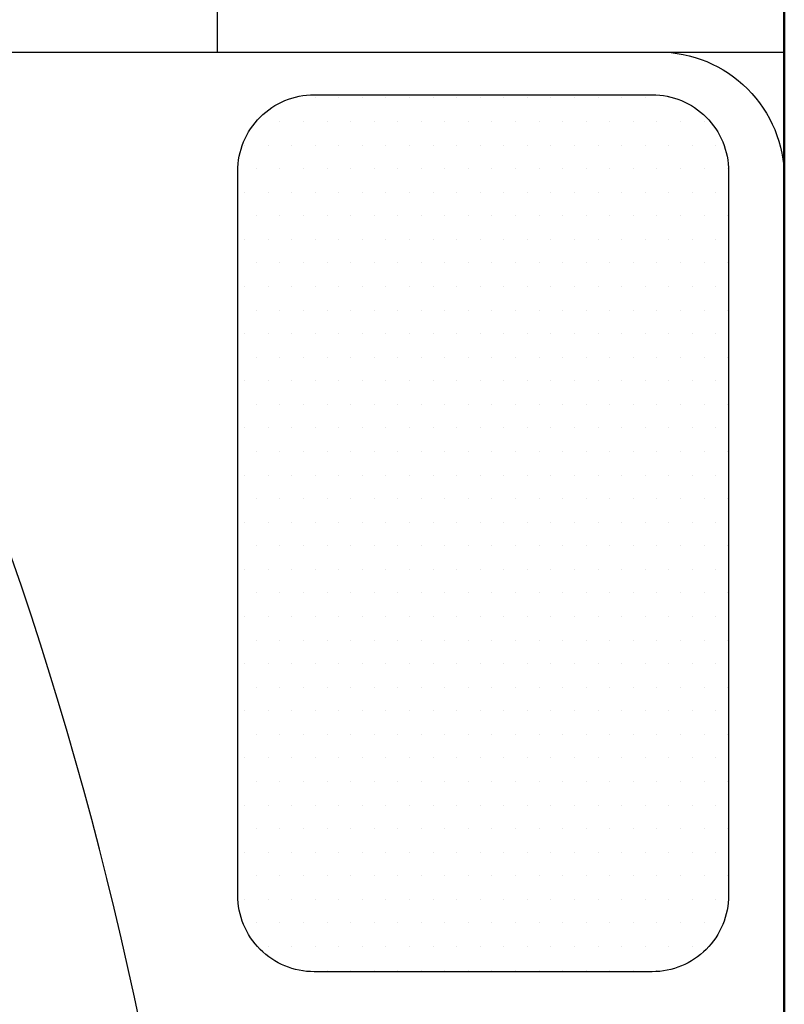
# Model space of a CAD drawing. Units: inches. Extents: x 3064 to 19385, y 846 to 15425.
# Tile 70 of 108: x 6580 to 6604, y 1655 to 1686. Entities that reach past the tile are written whole.
import ezdxf

# ---------------------------------------------------------------- set-up
doc = ezdxf.new("R2010")
doc.units = ezdxf.units.IN
doc.layers.add('A-FLOR-FIXT', color=9, linetype='Continuous', lineweight=18)
doc.layers.add('A-WALL', color=7, linetype='Continuous', lineweight=50)
doc.layers.add('BLOCK', color=6, linetype='Continuous')

# ---------------------------------------------------------------- blocks, each defined once
blk = doc.blocks.new('*X7')
at = {"color": 0}
for p, q in [((266.4375, 457.03125), (266.4375, 457.03125)), ((266.8125, 457.03125), (266.8125, 457.03125)), ((267.1875, 457.03125), (267.1875, 457.03125)), ((267.5625, 457.03125), (267.5625, 457.03125)), ((267.9375, 457.03125), (267.9375, 457.03125)), ((268.3125, 457.03125), (268.3125, 457.03125)), ((268.6875, 457.03125), (268.6875, 457.03125)), ((269.0625, 457.03125), (269.0625, 457.03125)), ((269.4375, 457.03125), (269.4375, 457.03125)), ((269.8125, 457.03125), (269.8125, 457.03125)), ((270.1875, 457.03125), (270.1875, 457.03125)), ((270.5625, 457.03125), (270.5625, 457.03125)), ((270.9375, 457.03125), (270.9375, 457.03125)), ((271.3125, 457.03125), (271.3125, 457.03125)), ((271.6875, 457.03125), (271.6875, 457.03125)), ((272.0625, 457.03125), (272.0625, 457.03125)), ((266.25, 456.9375), (266.25, 456.9375)), ((266.625, 456.9375), (266.625, 456.9375)), ((267, 456.9375), (267, 456.9375)), ((267.375, 456.9375), (267.375, 456.9375)), ((267.75, 456.9375), (267.75, 456.9375)), ((268.125, 456.9375), (268.125, 456.9375)), ((268.5, 456.9375), (268.5, 456.9375)), ((268.875, 456.9375), (268.875, 456.9375)), ((269.25, 456.9375), (269.25, 456.9375)), ((269.625, 456.9375), (269.625, 456.9375)), ((270, 456.9375), (270, 456.9375)), ((270.375, 456.9375), (270.375, 456.9375)), ((270.75, 456.9375), (270.75, 456.9375)), ((271.125, 456.9375), (271.125, 456.9375)), ((271.5, 456.9375), (271.5, 456.9375)), ((271.875, 456.9375), (271.875, 456.9375)), ((272.25, 456.9375), (272.25, 456.9375)), ((266.0625, 456.84375), (266.0625, 456.84375)), ((266.4375, 456.84375), (266.4375, 456.84375)), ((266.8125, 456.84375), (266.8125, 456.84375)), ((267.1875, 456.84375), (267.1875, 456.84375)), ((267.5625, 456.84375), (267.5625, 456.84375)), ((267.9375, 456.84375), (267.9375, 456.84375)), ((268.3125, 456.84375), (268.3125, 456.84375)), ((268.6875, 456.84375), (268.6875, 456.84375)), ((269.0625, 456.84375), (269.0625, 456.84375)), ((269.4375, 456.84375), (269.4375, 456.84375)), ((269.8125, 456.84375), (269.8125, 456.84375)), ((270.1875, 456.84375), (270.1875, 456.84375)), ((270.5625, 456.84375), (270.5625, 456.84375)), ((270.9375, 456.84375), (270.9375, 456.84375)), ((271.3125, 456.84375), (271.3125, 456.84375)), ((271.6875, 456.84375), (271.6875, 456.84375)), ((272.0625, 456.84375), (272.0625, 456.84375)), ((272.4375, 456.84375), (272.4375, 456.84375)), ((266.25, 456.75), (266.25, 456.75)), ((266.625, 456.75), (266.625, 456.75)), ((267, 456.75), (267, 456.75)), ((267.375, 456.75), (267.375, 456.75)), ((267.75, 456.75), (267.75, 456.75)), ((268.125, 456.75), (268.125, 456.75)), ((268.5, 456.75), (268.5, 456.75)), ((268.875, 456.75), (268.875, 456.75)), ((269.25, 456.75), (269.25, 456.75)), ((269.625, 456.75), (269.625, 456.75)), ((270, 456.75), (270, 456.75)), ((270.375, 456.75), (270.375, 456.75)), ((270.75, 456.75), (270.75, 456.75)), ((271.125, 456.75), (271.125, 456.75)), ((271.5, 456.75), (271.5, 456.75)), ((271.875, 456.75), (271.875, 456.75)), ((272.25, 456.75), (272.25, 456.75)), ((272.625, 456.75), (272.625, 456.75)), ((266.0625, 456.65625), (266.0625, 456.65625)), ((266.4375, 456.65625), (266.4375, 456.65625)), ((266.8125, 456.65625), (266.8125, 456.65625)), ((267.1875, 456.65625), (267.1875, 456.65625)), ((267.5625, 456.65625), (267.5625, 456.65625)), ((267.9375, 456.65625), (267.9375, 456.65625)), ((268.3125, 456.65625), (268.3125, 456.65625)), ((268.6875, 456.65625), (268.6875, 456.65625)), ((269.0625, 456.65625), (269.0625, 456.65625)), ((269.4375, 456.65625), (269.4375, 456.65625)), ((269.8125, 456.65625), (269.8125, 456.65625)), ((270.1875, 456.65625), (270.1875, 456.65625)), ((270.5625, 456.65625), (270.5625, 456.65625)), ((270.9375, 456.65625), (270.9375, 456.65625)), ((271.3125, 456.65625), (271.3125, 456.65625)), ((271.6875, 456.65625), (271.6875, 456.65625)), ((272.0625, 456.65625), (272.0625, 456.65625)), ((272.4375, 456.65625), (272.4375, 456.65625)), ((265.875, 456.5625), (265.875, 456.5625)), ((266.25, 456.5625), (266.25, 456.5625)), ((266.625, 456.5625), (266.625, 456.5625)), ((267, 456.5625), (267, 456.5625)), ((267.375, 456.5625), (267.375, 456.5625)), ((267.75, 456.5625), (267.75, 456.5625)), ((268.125, 456.5625), (268.125, 456.5625)), ((268.5, 456.5625), (268.5, 456.5625)), ((268.875, 456.5625), (268.875, 456.5625)), ((269.25, 456.5625), (269.25, 456.5625)), ((269.625, 456.5625), (269.625, 456.5625)), ((270, 456.5625), (270, 456.5625)), ((270.375, 456.5625), (270.375, 456.5625)), ((270.75, 456.5625), (270.75, 456.5625)), ((271.125, 456.5625), (271.125, 456.5625)), ((271.5, 456.5625), (271.5, 456.5625)), ((271.875, 456.5625), (271.875, 456.5625)), ((272.25, 456.5625), (272.25, 456.5625)), ((272.625, 456.5625), (272.625, 456.5625)), ((266.0625, 456.46875), (266.0625, 456.46875)), ((266.4375, 456.46875), (266.4375, 456.46875)), ((266.8125, 456.46875), (266.8125, 456.46875)), ((267.1875, 456.46875), (267.1875, 456.46875)), ((267.5625, 456.46875), (267.5625, 456.46875)), ((267.9375, 456.46875), (267.9375, 456.46875)), ((268.3125, 456.46875), (268.3125, 456.46875)), ((268.6875, 456.46875), (268.6875, 456.46875)), ((269.0625, 456.46875), (269.0625, 456.46875)), ((269.4375, 456.46875), (269.4375, 456.46875)), ((269.8125, 456.46875), (269.8125, 456.46875)), ((270.1875, 456.46875), (270.1875, 456.46875)), ((270.5625, 456.46875), (270.5625, 456.46875)), ((270.9375, 456.46875), (270.9375, 456.46875)), ((271.3125, 456.46875), (271.3125, 456.46875)), ((271.6875, 456.46875), (271.6875, 456.46875)), ((272.0625, 456.46875), (272.0625, 456.46875)), ((272.4375, 456.46875), (272.4375, 456.46875)), ((272.8125, 456.46875), (272.8125, 456.46875)), ((265.875, 456.375), (265.875, 456.375)), ((266.25, 456.375), (266.25, 456.375)), ((266.625, 456.375), (266.625, 456.375)), ((267, 456.375), (267, 456.375)), ((267.375, 456.375), (267.375, 456.375)), ((267.75, 456.375), (267.75, 456.375)), ((268.125, 456.375), (268.125, 456.375)), ((268.5, 456.375), (268.5, 456.375)), ((268.875, 456.375), (268.875, 456.375)), ((269.25, 456.375), (269.25, 456.375)), ((269.625, 456.375), (269.625, 456.375)), ((270, 456.375), (270, 456.375)), ((270.375, 456.375), (270.375, 456.375)), ((270.75, 456.375), (270.75, 456.375)), ((271.125, 456.375), (271.125, 456.375)), ((271.5, 456.375), (271.5, 456.375)), ((271.875, 456.375), (271.875, 456.375)), ((272.25, 456.375), (272.25, 456.375)), ((272.625, 456.375), (272.625, 456.375)), ((266.0625, 456.28125), (266.0625, 456.28125)), ((266.4375, 456.28125), (266.4375, 456.28125)), ((266.8125, 456.28125), (266.8125, 456.28125)), ((267.1875, 456.28125), (267.1875, 456.28125)), ((267.5625, 456.28125), (267.5625, 456.28125)), ((267.9375, 456.28125), (267.9375, 456.28125)), ((268.3125, 456.28125), (268.3125, 456.28125)), ((268.6875, 456.28125), (268.6875, 456.28125)), ((269.0625, 456.28125), (269.0625, 456.28125)), ((269.4375, 456.28125), (269.4375, 456.28125)), ((269.8125, 456.28125), (269.8125, 456.28125)), ((270.1875, 456.28125), (270.1875, 456.28125)), ((270.5625, 456.28125), (270.5625, 456.28125)), ((270.9375, 456.28125), (270.9375, 456.28125)), ((271.3125, 456.28125), (271.3125, 456.28125)), ((271.6875, 456.28125), (271.6875, 456.28125)), ((272.0625, 456.28125), (272.0625, 456.28125)), ((272.4375, 456.28125), (272.4375, 456.28125)), ((272.8125, 456.28125), (272.8125, 456.28125)), ((265.875, 456.1875), (265.875, 456.1875)), ((266.25, 456.1875), (266.25, 456.1875)), ((266.625, 456.1875), (266.625, 456.1875)), ((267, 456.1875), (267, 456.1875)), ((267.375, 456.1875), (267.375, 456.1875)), ((267.75, 456.1875), (267.75, 456.1875)), ((268.125, 456.1875), (268.125, 456.1875)), ((268.5, 456.1875), (268.5, 456.1875)), ((268.875, 456.1875), (268.875, 456.1875)), ((269.25, 456.1875), (269.25, 456.1875)), ((269.625, 456.1875), (269.625, 456.1875)), ((270, 456.1875), (270, 456.1875)), ((270.375, 456.1875), (270.375, 456.1875)), ((270.75, 456.1875), (270.75, 456.1875)), ((271.125, 456.1875), (271.125, 456.1875)), ((271.5, 456.1875), (271.5, 456.1875)), ((271.875, 456.1875), (271.875, 456.1875)), ((272.25, 456.1875), (272.25, 456.1875)), ((272.625, 456.1875), (272.625, 456.1875)), ((266.0625, 456.09375), (266.0625, 456.09375)), ((266.4375, 456.09375), (266.4375, 456.09375)), ((266.8125, 456.09375), (266.8125, 456.09375)), ((267.1875, 456.09375), (267.1875, 456.09375)), ((267.5625, 456.09375), (267.5625, 456.09375)), ((267.9375, 456.09375), (267.9375, 456.09375)), ((268.3125, 456.09375), (268.3125, 456.09375)), ((268.6875, 456.09375), (268.6875, 456.09375)), ((269.0625, 456.09375), (269.0625, 456.09375)), ((269.4375, 456.09375), (269.4375, 456.09375)), ((269.8125, 456.09375), (269.8125, 456.09375)), ((270.1875, 456.09375), (270.1875, 456.09375)), ((270.5625, 456.09375), (270.5625, 456.09375)), ((270.9375, 456.09375), (270.9375, 456.09375)), ((271.3125, 456.09375), (271.3125, 456.09375)), ((271.6875, 456.09375), (271.6875, 456.09375)), ((272.0625, 456.09375), (272.0625, 456.09375)), ((272.4375, 456.09375), (272.4375, 456.09375)), ((272.8125, 456.09375), (272.8125, 456.09375)), ((265.875, 456), (265.875, 456)), ((266.25, 456), (266.25, 456)), ((266.625, 456), (266.625, 456)), ((267, 456), (267, 456)), ((267.375, 456), (267.375, 456)), ((267.75, 456), (267.75, 456)), ((268.125, 456), (268.125, 456)), ((268.5, 456), (268.5, 456)), ((268.875, 456), (268.875, 456)), ((269.25, 456), (269.25, 456)), ((269.625, 456), (269.625, 456)), ((270, 456), (270, 456)), ((270.375, 456), (270.375, 456)), ((270.75, 456), (270.75, 456)), ((271.125, 456), (271.125, 456)), ((271.5, 456), (271.5, 456)), ((271.875, 456), (271.875, 456)), ((272.25, 456), (272.25, 456)), ((272.625, 456), (272.625, 456)), ((266.0625, 455.90625), (266.0625, 455.90625)), ((266.4375, 455.90625), (266.4375, 455.90625)), ((266.8125, 455.90625), (266.8125, 455.90625)), ((267.1875, 455.90625), (267.1875, 455.90625)), ((267.5625, 455.90625), (267.5625, 455.90625)), ((267.9375, 455.90625), (267.9375, 455.90625)), ((268.3125, 455.90625), (268.3125, 455.90625)), ((268.6875, 455.90625), (268.6875, 455.90625)), ((269.0625, 455.90625), (269.0625, 455.90625)), ((269.4375, 455.90625), (269.4375, 455.90625)), ((269.8125, 455.90625), (269.8125, 455.90625)), ((270.1875, 455.90625), (270.1875, 455.90625)), ((270.5625, 455.90625), (270.5625, 455.90625)), ((270.9375, 455.90625), (270.9375, 455.90625)), ((271.3125, 455.90625), (271.3125, 455.90625)), ((271.6875, 455.90625), (271.6875, 455.90625)), ((272.0625, 455.90625), (272.0625, 455.90625)), ((272.4375, 455.90625), (272.4375, 455.90625)), ((272.8125, 455.90625), (272.8125, 455.90625)), ((265.875, 455.8125), (265.875, 455.8125)), ((266.25, 455.8125), (266.25, 455.8125)), ((266.625, 455.8125), (266.625, 455.8125)), ((267, 455.8125), (267, 455.8125)), ((267.375, 455.8125), (267.375, 455.8125)), ((267.75, 455.8125), (267.75, 455.8125)), ((268.125, 455.8125), (268.125, 455.8125)), ((268.5, 455.8125), (268.5, 455.8125)), ((268.875, 455.8125), (268.875, 455.8125)), ((269.25, 455.8125), (269.25, 455.8125)), ((269.625, 455.8125), (269.625, 455.8125)), ((270, 455.8125), (270, 455.8125)), ((270.375, 455.8125), (270.375, 455.8125)), ((270.75, 455.8125), (270.75, 455.8125)), ((271.125, 455.8125), (271.125, 455.8125)), ((271.5, 455.8125), (271.5, 455.8125)), ((271.875, 455.8125), (271.875, 455.8125)), ((272.25, 455.8125), (272.25, 455.8125)), ((272.625, 455.8125), (272.625, 455.8125)), ((266.0625, 455.71875), (266.0625, 455.71875)), ((266.4375, 455.71875), (266.4375, 455.71875)), ((266.8125, 455.71875), (266.8125, 455.71875)), ((267.1875, 455.71875), (267.1875, 455.71875)), ((267.5625, 455.71875), (267.5625, 455.71875)), ((267.9375, 455.71875), (267.9375, 455.71875)), ((268.3125, 455.71875), (268.3125, 455.71875)), ((268.6875, 455.71875), (268.6875, 455.71875)), ((269.0625, 455.71875), (269.0625, 455.71875)), ((269.4375, 455.71875), (269.4375, 455.71875)), ((269.8125, 455.71875), (269.8125, 455.71875)), ((270.1875, 455.71875), (270.1875, 455.71875)), ((270.5625, 455.71875), (270.5625, 455.71875)), ((270.9375, 455.71875), (270.9375, 455.71875)), ((271.3125, 455.71875), (271.3125, 455.71875)), ((271.6875, 455.71875), (271.6875, 455.71875)), ((272.0625, 455.71875), (272.0625, 455.71875)), ((272.4375, 455.71875), (272.4375, 455.71875)), ((272.8125, 455.71875), (272.8125, 455.71875)), ((265.875, 455.625), (265.875, 455.625)), ((266.25, 455.625), (266.25, 455.625)), ((266.625, 455.625), (266.625, 455.625)), ((267, 455.625), (267, 455.625)), ((267.375, 455.625), (267.375, 455.625)), ((267.75, 455.625), (267.75, 455.625)), ((268.125, 455.625), (268.125, 455.625)), ((268.5, 455.625), (268.5, 455.625)), ((268.875, 455.625), (268.875, 455.625)), ((269.25, 455.625), (269.25, 455.625)), ((269.625, 455.625), (269.625, 455.625)), ((270, 455.625), (270, 455.625)), ((270.375, 455.625), (270.375, 455.625)), ((270.75, 455.625), (270.75, 455.625)), ((271.125, 455.625), (271.125, 455.625)), ((271.5, 455.625), (271.5, 455.625)), ((271.875, 455.625), (271.875, 455.625)), ((272.25, 455.625), (272.25, 455.625)), ((272.625, 455.625), (272.625, 455.625)), ((266.0625, 455.53125), (266.0625, 455.53125)), ((266.4375, 455.53125), (266.4375, 455.53125)), ((266.8125, 455.53125), (266.8125, 455.53125)), ((267.1875, 455.53125), (267.1875, 455.53125)), ((267.5625, 455.53125), (267.5625, 455.53125)), ((267.9375, 455.53125), (267.9375, 455.53125)), ((268.3125, 455.53125), (268.3125, 455.53125)), ((268.6875, 455.53125), (268.6875, 455.53125)), ((269.0625, 455.53125), (269.0625, 455.53125)), ((269.4375, 455.53125), (269.4375, 455.53125)), ((269.8125, 455.53125), (269.8125, 455.53125)), ((270.1875, 455.53125), (270.1875, 455.53125)), ((270.5625, 455.53125), (270.5625, 455.53125)), ((270.9375, 455.53125), (270.9375, 455.53125)), ((271.3125, 455.53125), (271.3125, 455.53125)), ((271.6875, 455.53125), (271.6875, 455.53125)), ((272.0625, 455.53125), (272.0625, 455.53125)), ((272.4375, 455.53125), (272.4375, 455.53125)), ((272.8125, 455.53125), (272.8125, 455.53125)), ((265.875, 455.4375), (265.875, 455.4375)), ((266.25, 455.4375), (266.25, 455.4375)), ((266.625, 455.4375), (266.625, 455.4375)), ((267, 455.4375), (267, 455.4375)), ((267.375, 455.4375), (267.375, 455.4375)), ((267.75, 455.4375), (267.75, 455.4375)), ((268.125, 455.4375), (268.125, 455.4375)), ((268.5, 455.4375), (268.5, 455.4375)), ((268.875, 455.4375), (268.875, 455.4375)), ((269.25, 455.4375), (269.25, 455.4375)), ((269.625, 455.4375), (269.625, 455.4375)), ((270, 455.4375), (270, 455.4375)), ((270.375, 455.4375), (270.375, 455.4375)), ((270.75, 455.4375), (270.75, 455.4375)), ((271.125, 455.4375), (271.125, 455.4375)), ((271.5, 455.4375), (271.5, 455.4375)), ((271.875, 455.4375), (271.875, 455.4375)), ((272.25, 455.4375), (272.25, 455.4375)), ((272.625, 455.4375), (272.625, 455.4375)), ((266.0625, 455.34375), (266.0625, 455.34375)), ((266.4375, 455.34375), (266.4375, 455.34375)), ((266.8125, 455.34375), (266.8125, 455.34375)), ((267.1875, 455.34375), (267.1875, 455.34375)), ((267.5625, 455.34375), (267.5625, 455.34375)), ((267.9375, 455.34375), (267.9375, 455.34375)), ((268.3125, 455.34375), (268.3125, 455.34375)), ((268.6875, 455.34375), (268.6875, 455.34375)), ((269.0625, 455.34375), (269.0625, 455.34375)), ((269.4375, 455.34375), (269.4375, 455.34375)), ((269.8125, 455.34375), (269.8125, 455.34375)), ((270.1875, 455.34375), (270.1875, 455.34375)), ((270.5625, 455.34375), (270.5625, 455.34375)), ((270.9375, 455.34375), (270.9375, 455.34375)), ((271.3125, 455.34375), (271.3125, 455.34375)), ((271.6875, 455.34375), (271.6875, 455.34375)), ((272.0625, 455.34375), (272.0625, 455.34375)), ((272.4375, 455.34375), (272.4375, 455.34375)), ((272.8125, 455.34375), (272.8125, 455.34375)), ((265.875, 455.25), (265.875, 455.25)), ((266.25, 455.25), (266.25, 455.25)), ((266.625, 455.25), (266.625, 455.25)), ((267, 455.25), (267, 455.25)), ((267.375, 455.25), (267.375, 455.25)), ((267.75, 455.25), (267.75, 455.25)), ((268.125, 455.25), (268.125, 455.25)), ((268.5, 455.25), (268.5, 455.25)), ((268.875, 455.25), (268.875, 455.25)), ((269.25, 455.25), (269.25, 455.25)), ((269.625, 455.25), (269.625, 455.25)), ((270, 455.25), (270, 455.25)), ((270.375, 455.25), (270.375, 455.25)), ((270.75, 455.25), (270.75, 455.25)), ((271.125, 455.25), (271.125, 455.25)), ((271.5, 455.25), (271.5, 455.25)), ((271.875, 455.25), (271.875, 455.25)), ((272.25, 455.25), (272.25, 455.25)), ((272.625, 455.25), (272.625, 455.25)), ((266.0625, 455.15625), (266.0625, 455.15625)), ((266.4375, 455.15625), (266.4375, 455.15625)), ((266.8125, 455.15625), (266.8125, 455.15625)), ((267.1875, 455.15625), (267.1875, 455.15625)), ((267.5625, 455.15625), (267.5625, 455.15625)), ((267.9375, 455.15625), (267.9375, 455.15625)), ((268.3125, 455.15625), (268.3125, 455.15625)), ((268.6875, 455.15625), (268.6875, 455.15625)), ((269.0625, 455.15625), (269.0625, 455.15625)), ((269.4375, 455.15625), (269.4375, 455.15625)), ((269.8125, 455.15625), (269.8125, 455.15625)), ((270.1875, 455.15625), (270.1875, 455.15625)), ((270.5625, 455.15625), (270.5625, 455.15625)), ((270.9375, 455.15625), (270.9375, 455.15625)), ((271.3125, 455.15625), (271.3125, 455.15625)), ((271.6875, 455.15625), (271.6875, 455.15625)), ((272.0625, 455.15625), (272.0625, 455.15625)), ((272.4375, 455.15625), (272.4375, 455.15625)), ((272.8125, 455.15625), (272.8125, 455.15625)), ((265.875, 455.0625), (265.875, 455.0625)), ((266.25, 455.0625), (266.25, 455.0625)), ((266.625, 455.0625), (266.625, 455.0625)), ((267, 455.0625), (267, 455.0625)), ((267.375, 455.0625), (267.375, 455.0625)), ((267.75, 455.0625), (267.75, 455.0625)), ((268.125, 455.0625), (268.125, 455.0625)), ((268.5, 455.0625), (268.5, 455.0625)), ((268.875, 455.0625), (268.875, 455.0625)), ((269.25, 455.0625), (269.25, 455.0625)), ((269.625, 455.0625), (269.625, 455.0625)), ((270, 455.0625), (270, 455.0625)), ((270.375, 455.0625), (270.375, 455.0625)), ((270.75, 455.0625), (270.75, 455.0625)), ((271.125, 455.0625), (271.125, 455.0625)), ((271.5, 455.0625), (271.5, 455.0625)), ((271.875, 455.0625), (271.875, 455.0625)), ((272.25, 455.0625), (272.25, 455.0625)), ((272.625, 455.0625), (272.625, 455.0625)), ((266.0625, 454.96875), (266.0625, 454.96875)), ((266.4375, 454.96875), (266.4375, 454.96875)), ((266.8125, 454.96875), (266.8125, 454.96875)), ((267.1875, 454.96875), (267.1875, 454.96875)), ((267.5625, 454.96875), (267.5625, 454.96875)), ((267.9375, 454.96875), (267.9375, 454.96875)), ((268.3125, 454.96875), (268.3125, 454.96875)), ((268.6875, 454.96875), (268.6875, 454.96875)), ((269.0625, 454.96875), (269.0625, 454.96875)), ((269.4375, 454.96875), (269.4375, 454.96875)), ((269.8125, 454.96875), (269.8125, 454.96875)), ((270.1875, 454.96875), (270.1875, 454.96875)), ((270.5625, 454.96875), (270.5625, 454.96875)), ((270.9375, 454.96875), (270.9375, 454.96875)), ((271.3125, 454.96875), (271.3125, 454.96875)), ((271.6875, 454.96875), (271.6875, 454.96875)), ((272.0625, 454.96875), (272.0625, 454.96875)), ((272.4375, 454.96875), (272.4375, 454.96875)), ((272.8125, 454.96875), (272.8125, 454.96875)), ((265.875, 454.875), (265.875, 454.875)), ((266.25, 454.875), (266.25, 454.875)), ((266.625, 454.875), (266.625, 454.875)), ((267, 454.875), (267, 454.875)), ((267.375, 454.875), (267.375, 454.875)), ((267.75, 454.875), (267.75, 454.875)), ((268.125, 454.875), (268.125, 454.875)), ((268.5, 454.875), (268.5, 454.875)), ((268.875, 454.875), (268.875, 454.875)), ((269.25, 454.875), (269.25, 454.875)), ((269.625, 454.875), (269.625, 454.875)), ((270, 454.875), (270, 454.875)), ((270.375, 454.875), (270.375, 454.875)), ((270.75, 454.875), (270.75, 454.875)), ((271.125, 454.875), (271.125, 454.875)), ((271.5, 454.875), (271.5, 454.875)), ((271.875, 454.875), (271.875, 454.875)), ((272.25, 454.875), (272.25, 454.875)), ((272.625, 454.875), (272.625, 454.875)), ((266.0625, 454.78125), (266.0625, 454.78125)), ((266.4375, 454.78125), (266.4375, 454.78125)), ((266.8125, 454.78125), (266.8125, 454.78125)), ((267.1875, 454.78125), (267.1875, 454.78125)), ((267.5625, 454.78125), (267.5625, 454.78125)), ((267.9375, 454.78125), (267.9375, 454.78125)), ((268.3125, 454.78125), (268.3125, 454.78125)), ((268.6875, 454.78125), (268.6875, 454.78125)), ((269.0625, 454.78125), (269.0625, 454.78125)), ((269.4375, 454.78125), (269.4375, 454.78125)), ((269.8125, 454.78125), (269.8125, 454.78125)), ((270.1875, 454.78125), (270.1875, 454.78125)), ((270.5625, 454.78125), (270.5625, 454.78125)), ((270.9375, 454.78125), (270.9375, 454.78125)), ((271.3125, 454.78125), (271.3125, 454.78125)), ((271.6875, 454.78125), (271.6875, 454.78125)), ((272.0625, 454.78125), (272.0625, 454.78125)), ((272.4375, 454.78125), (272.4375, 454.78125)), ((272.8125, 454.78125), (272.8125, 454.78125)), ((265.875, 454.6875), (265.875, 454.6875)), ((266.25, 454.6875), (266.25, 454.6875)), ((266.625, 454.6875), (266.625, 454.6875)), ((267, 454.6875), (267, 454.6875)), ((267.375, 454.6875), (267.375, 454.6875)), ((267.75, 454.6875), (267.75, 454.6875)), ((268.125, 454.6875), (268.125, 454.6875)), ((268.5, 454.6875), (268.5, 454.6875)), ((268.875, 454.6875), (268.875, 454.6875)), ((269.25, 454.6875), (269.25, 454.6875)), ((269.625, 454.6875), (269.625, 454.6875)), ((270, 454.6875), (270, 454.6875)), ((270.375, 454.6875), (270.375, 454.6875)), ((270.75, 454.6875), (270.75, 454.6875)), ((271.125, 454.6875), (271.125, 454.6875)), ((271.5, 454.6875), (271.5, 454.6875)), ((271.875, 454.6875), (271.875, 454.6875)), ((272.25, 454.6875), (272.25, 454.6875)), ((272.625, 454.6875), (272.625, 454.6875)), ((266.0625, 454.59375), (266.0625, 454.59375)), ((266.4375, 454.59375), (266.4375, 454.59375)), ((266.8125, 454.59375), (266.8125, 454.59375)), ((267.1875, 454.59375), (267.1875, 454.59375)), ((267.5625, 454.59375), (267.5625, 454.59375)), ((267.9375, 454.59375), (267.9375, 454.59375)), ((268.3125, 454.59375), (268.3125, 454.59375)), ((268.6875, 454.59375), (268.6875, 454.59375)), ((269.0625, 454.59375), (269.0625, 454.59375)), ((269.4375, 454.59375), (269.4375, 454.59375)), ((269.8125, 454.59375), (269.8125, 454.59375)), ((270.1875, 454.59375), (270.1875, 454.59375)), ((270.5625, 454.59375), (270.5625, 454.59375)), ((270.9375, 454.59375), (270.9375, 454.59375)), ((271.3125, 454.59375), (271.3125, 454.59375)), ((271.6875, 454.59375), (271.6875, 454.59375)), ((272.0625, 454.59375), (272.0625, 454.59375)), ((272.4375, 454.59375), (272.4375, 454.59375)), ((272.8125, 454.59375), (272.8125, 454.59375)), ((265.875, 454.5), (265.875, 454.5)), ((266.25, 454.5), (266.25, 454.5)), ((266.625, 454.5), (266.625, 454.5)), ((267, 454.5), (267, 454.5)), ((267.375, 454.5), (267.375, 454.5)), ((267.75, 454.5), (267.75, 454.5)), ((268.125, 454.5), (268.125, 454.5)), ((268.5, 454.5), (268.5, 454.5)), ((268.875, 454.5), (268.875, 454.5)), ((269.25, 454.5), (269.25, 454.5)), ((269.625, 454.5), (269.625, 454.5)), ((270, 454.5), (270, 454.5)), ((270.375, 454.5), (270.375, 454.5)), ((270.75, 454.5), (270.75, 454.5)), ((271.125, 454.5), (271.125, 454.5)), ((271.5, 454.5), (271.5, 454.5)), ((271.875, 454.5), (271.875, 454.5)), ((272.25, 454.5), (272.25, 454.5)), ((272.625, 454.5), (272.625, 454.5)), ((266.0625, 454.40625), (266.0625, 454.40625)), ((266.4375, 454.40625), (266.4375, 454.40625)), ((266.8125, 454.40625), (266.8125, 454.40625)), ((267.1875, 454.40625), (267.1875, 454.40625)), ((267.5625, 454.40625), (267.5625, 454.40625)), ((267.9375, 454.40625), (267.9375, 454.40625)), ((268.3125, 454.40625), (268.3125, 454.40625)), ((268.6875, 454.40625), (268.6875, 454.40625)), ((269.0625, 454.40625), (269.0625, 454.40625)), ((269.4375, 454.40625), (269.4375, 454.40625)), ((269.8125, 454.40625), (269.8125, 454.40625)), ((270.1875, 454.40625), (270.1875, 454.40625)), ((270.5625, 454.40625), (270.5625, 454.40625)), ((270.9375, 454.40625), (270.9375, 454.40625)), ((271.3125, 454.40625), (271.3125, 454.40625)), ((271.6875, 454.40625), (271.6875, 454.40625)), ((272.0625, 454.40625), (272.0625, 454.40625)), ((272.4375, 454.40625), (272.4375, 454.40625)), ((272.8125, 454.40625), (272.8125, 454.40625)), ((265.875, 454.3125), (265.875, 454.3125)), ((266.25, 454.3125), (266.25, 454.3125)), ((266.625, 454.3125), (266.625, 454.3125)), ((267, 454.3125), (267, 454.3125)), ((267.375, 454.3125), (267.375, 454.3125)), ((267.75, 454.3125), (267.75, 454.3125)), ((268.125, 454.3125), (268.125, 454.3125)), ((268.5, 454.3125), (268.5, 454.3125)), ((268.875, 454.3125), (268.875, 454.3125)), ((269.25, 454.3125), (269.25, 454.3125)), ((269.625, 454.3125), (269.625, 454.3125)), ((270, 454.3125), (270, 454.3125)), ((270.375, 454.3125), (270.375, 454.3125)), ((270.75, 454.3125), (270.75, 454.3125)), ((271.125, 454.3125), (271.125, 454.3125)), ((271.5, 454.3125), (271.5, 454.3125)), ((271.875, 454.3125), (271.875, 454.3125)), ((272.25, 454.3125), (272.25, 454.3125)), ((272.625, 454.3125), (272.625, 454.3125)), ((266.0625, 454.21875), (266.0625, 454.21875)), ((266.4375, 454.21875), (266.4375, 454.21875)), ((266.8125, 454.21875), (266.8125, 454.21875)), ((267.1875, 454.21875), (267.1875, 454.21875)), ((267.5625, 454.21875), (267.5625, 454.21875)), ((267.9375, 454.21875), (267.9375, 454.21875)), ((268.3125, 454.21875), (268.3125, 454.21875)), ((268.6875, 454.21875), (268.6875, 454.21875)), ((269.0625, 454.21875), (269.0625, 454.21875)), ((269.4375, 454.21875), (269.4375, 454.21875)), ((269.8125, 454.21875), (269.8125, 454.21875)), ((270.1875, 454.21875), (270.1875, 454.21875)), ((270.5625, 454.21875), (270.5625, 454.21875)), ((270.9375, 454.21875), (270.9375, 454.21875)), ((271.3125, 454.21875), (271.3125, 454.21875)), ((271.6875, 454.21875), (271.6875, 454.21875)), ((272.0625, 454.21875), (272.0625, 454.21875)), ((272.4375, 454.21875), (272.4375, 454.21875)), ((272.8125, 454.21875), (272.8125, 454.21875)), ((265.875, 454.125), (265.875, 454.125)), ((266.25, 454.125), (266.25, 454.125)), ((266.625, 454.125), (266.625, 454.125)), ((267, 454.125), (267, 454.125)), ((267.375, 454.125), (267.375, 454.125)), ((267.75, 454.125), (267.75, 454.125)), ((268.125, 454.125), (268.125, 454.125)), ((268.5, 454.125), (268.5, 454.125)), ((268.875, 454.125), (268.875, 454.125)), ((269.25, 454.125), (269.25, 454.125)), ((269.625, 454.125), (269.625, 454.125)), ((270, 454.125), (270, 454.125)), ((270.375, 454.125), (270.375, 454.125)), ((270.75, 454.125), (270.75, 454.125)), ((271.125, 454.125), (271.125, 454.125)), ((271.5, 454.125), (271.5, 454.125)), ((271.875, 454.125), (271.875, 454.125)), ((272.25, 454.125), (272.25, 454.125)), ((272.625, 454.125), (272.625, 454.125)), ((266.0625, 454.03125), (266.0625, 454.03125)), ((266.4375, 454.03125), (266.4375, 454.03125)), ((266.8125, 454.03125), (266.8125, 454.03125)), ((267.1875, 454.03125), (267.1875, 454.03125)), ((267.5625, 454.03125), (267.5625, 454.03125)), ((267.9375, 454.03125), (267.9375, 454.03125)), ((268.3125, 454.03125), (268.3125, 454.03125)), ((268.6875, 454.03125), (268.6875, 454.03125)), ((269.0625, 454.03125), (269.0625, 454.03125)), ((269.4375, 454.03125), (269.4375, 454.03125)), ((269.8125, 454.03125), (269.8125, 454.03125)), ((270.1875, 454.03125), (270.1875, 454.03125)), ((270.5625, 454.03125), (270.5625, 454.03125)), ((270.9375, 454.03125), (270.9375, 454.03125)), ((271.3125, 454.03125), (271.3125, 454.03125)), ((271.6875, 454.03125), (271.6875, 454.03125)), ((272.0625, 454.03125), (272.0625, 454.03125)), ((272.4375, 454.03125), (272.4375, 454.03125)), ((272.8125, 454.03125), (272.8125, 454.03125)), ((265.875, 453.9375), (265.875, 453.9375)), ((266.25, 453.9375), (266.25, 453.9375)), ((266.625, 453.9375), (266.625, 453.9375)), ((267, 453.9375), (267, 453.9375)), ((267.375, 453.9375), (267.375, 453.9375)), ((267.75, 453.9375), (267.75, 453.9375)), ((268.125, 453.9375), (268.125, 453.9375)), ((268.5, 453.9375), (268.5, 453.9375)), ((268.875, 453.9375), (268.875, 453.9375)), ((269.25, 453.9375), (269.25, 453.9375)), ((269.625, 453.9375), (269.625, 453.9375)), ((270, 453.9375), (270, 453.9375)), ((270.375, 453.9375), (270.375, 453.9375)), ((270.75, 453.9375), (270.75, 453.9375)), ((271.125, 453.9375), (271.125, 453.9375)), ((271.5, 453.9375), (271.5, 453.9375)), ((271.875, 453.9375), (271.875, 453.9375)), ((272.25, 453.9375), (272.25, 453.9375)), ((272.625, 453.9375), (272.625, 453.9375)), ((266.0625, 453.84375), (266.0625, 453.84375)), ((266.4375, 453.84375), (266.4375, 453.84375)), ((266.8125, 453.84375), (266.8125, 453.84375)), ((267.1875, 453.84375), (267.1875, 453.84375)), ((267.5625, 453.84375), (267.5625, 453.84375)), ((267.9375, 453.84375), (267.9375, 453.84375)), ((268.3125, 453.84375), (268.3125, 453.84375)), ((268.6875, 453.84375), (268.6875, 453.84375)), ((269.0625, 453.84375), (269.0625, 453.84375)), ((269.4375, 453.84375), (269.4375, 453.84375)), ((269.8125, 453.84375), (269.8125, 453.84375)), ((270.1875, 453.84375), (270.1875, 453.84375)), ((270.5625, 453.84375), (270.5625, 453.84375)), ((270.9375, 453.84375), (270.9375, 453.84375)), ((271.3125, 453.84375), (271.3125, 453.84375)), ((271.6875, 453.84375), (271.6875, 453.84375)), ((272.0625, 453.84375), (272.0625, 453.84375)), ((272.4375, 453.84375), (272.4375, 453.84375)), ((272.8125, 453.84375), (272.8125, 453.84375)), ((265.875, 453.75), (265.875, 453.75)), ((266.25, 453.75), (266.25, 453.75)), ((266.625, 453.75), (266.625, 453.75)), ((267, 453.75), (267, 453.75)), ((267.375, 453.75), (267.375, 453.75)), ((267.75, 453.75), (267.75, 453.75)), ((268.125, 453.75), (268.125, 453.75)), ((268.5, 453.75), (268.5, 453.75)), ((268.875, 453.75), (268.875, 453.75)), ((269.25, 453.75), (269.25, 453.75)), ((269.625, 453.75), (269.625, 453.75)), ((270, 453.75), (270, 453.75)), ((270.375, 453.75), (270.375, 453.75)), ((270.75, 453.75), (270.75, 453.75)), ((271.125, 453.75), (271.125, 453.75)), ((271.5, 453.75), (271.5, 453.75)), ((271.875, 453.75), (271.875, 453.75)), ((272.25, 453.75), (272.25, 453.75)), ((272.625, 453.75), (272.625, 453.75)), ((266.0625, 453.65625), (266.0625, 453.65625)), ((266.4375, 453.65625), (266.4375, 453.65625)), ((266.8125, 453.65625), (266.8125, 453.65625)), ((267.1875, 453.65625), (267.1875, 453.65625)), ((267.5625, 453.65625), (267.5625, 453.65625)), ((267.9375, 453.65625), (267.9375, 453.65625)), ((268.3125, 453.65625), (268.3125, 453.65625)), ((268.6875, 453.65625), (268.6875, 453.65625)), ((269.0625, 453.65625), (269.0625, 453.65625)), ((269.4375, 453.65625), (269.4375, 453.65625)), ((269.8125, 453.65625), (269.8125, 453.65625)), ((270.1875, 453.65625), (270.1875, 453.65625)), ((270.5625, 453.65625), (270.5625, 453.65625)), ((270.9375, 453.65625), (270.9375, 453.65625)), ((271.3125, 453.65625), (271.3125, 453.65625)), ((271.6875, 453.65625), (271.6875, 453.65625)), ((272.0625, 453.65625), (272.0625, 453.65625)), ((272.4375, 453.65625), (272.4375, 453.65625)), ((272.8125, 453.65625), (272.8125, 453.65625)), ((266.25, 453.5625), (266.25, 453.5625)), ((266.625, 453.5625), (266.625, 453.5625)), ((267, 453.5625), (267, 453.5625)), ((267.375, 453.5625), (267.375, 453.5625)), ((267.75, 453.5625), (267.75, 453.5625)), ((268.125, 453.5625), (268.125, 453.5625)), ((268.5, 453.5625), (268.5, 453.5625)), ((268.875, 453.5625), (268.875, 453.5625)), ((269.25, 453.5625), (269.25, 453.5625)), ((269.625, 453.5625), (269.625, 453.5625)), ((270, 453.5625), (270, 453.5625)), ((270.375, 453.5625), (270.375, 453.5625)), ((270.75, 453.5625), (270.75, 453.5625)), ((271.125, 453.5625), (271.125, 453.5625)), ((271.5, 453.5625), (271.5, 453.5625)), ((271.875, 453.5625), (271.875, 453.5625)), ((272.25, 453.5625), (272.25, 453.5625)), ((272.625, 453.5625), (272.625, 453.5625)), ((266.0625, 453.46875), (266.0625, 453.46875)), ((266.4375, 453.46875), (266.4375, 453.46875)), ((266.8125, 453.46875), (266.8125, 453.46875)), ((267.1875, 453.46875), (267.1875, 453.46875)), ((267.5625, 453.46875), (267.5625, 453.46875)), ((267.9375, 453.46875), (267.9375, 453.46875)), ((268.3125, 453.46875), (268.3125, 453.46875)), ((268.6875, 453.46875), (268.6875, 453.46875)), ((269.0625, 453.46875), (269.0625, 453.46875)), ((269.4375, 453.46875), (269.4375, 453.46875)), ((269.8125, 453.46875), (269.8125, 453.46875)), ((270.1875, 453.46875), (270.1875, 453.46875)), ((270.5625, 453.46875), (270.5625, 453.46875)), ((270.9375, 453.46875), (270.9375, 453.46875)), ((271.3125, 453.46875), (271.3125, 453.46875)), ((271.6875, 453.46875), (271.6875, 453.46875)), ((272.0625, 453.46875), (272.0625, 453.46875)), ((272.4375, 453.46875), (272.4375, 453.46875)), ((266.25, 453.375), (266.25, 453.375)), ((266.625, 453.375), (266.625, 453.375)), ((267, 453.375), (267, 453.375)), ((267.375, 453.375), (267.375, 453.375)), ((267.75, 453.375), (267.75, 453.375)), ((268.125, 453.375), (268.125, 453.375)), ((268.5, 453.375), (268.5, 453.375)), ((268.875, 453.375), (268.875, 453.375)), ((269.25, 453.375), (269.25, 453.375)), ((269.625, 453.375), (269.625, 453.375)), ((270, 453.375), (270, 453.375)), ((270.375, 453.375), (270.375, 453.375)), ((270.75, 453.375), (270.75, 453.375)), ((271.125, 453.375), (271.125, 453.375)), ((271.5, 453.375), (271.5, 453.375)), ((271.875, 453.375), (271.875, 453.375)), ((272.25, 453.375), (272.25, 453.375)), ((272.625, 453.375), (272.625, 453.375)), ((266.0625, 453.28125), (266.0625, 453.28125)), ((266.4375, 453.28125), (266.4375, 453.28125)), ((266.8125, 453.28125), (266.8125, 453.28125)), ((267.1875, 453.28125), (267.1875, 453.28125)), ((267.5625, 453.28125), (267.5625, 453.28125)), ((267.9375, 453.28125), (267.9375, 453.28125)), ((268.3125, 453.28125), (268.3125, 453.28125)), ((268.6875, 453.28125), (268.6875, 453.28125)), ((269.0625, 453.28125), (269.0625, 453.28125)), ((269.4375, 453.28125), (269.4375, 453.28125)), ((269.8125, 453.28125), (269.8125, 453.28125)), ((270.1875, 453.28125), (270.1875, 453.28125)), ((270.5625, 453.28125), (270.5625, 453.28125)), ((270.9375, 453.28125), (270.9375, 453.28125)), ((271.3125, 453.28125), (271.3125, 453.28125)), ((271.6875, 453.28125), (271.6875, 453.28125)), ((272.0625, 453.28125), (272.0625, 453.28125)), ((272.4375, 453.28125), (272.4375, 453.28125)), ((266.25, 453.1875), (266.25, 453.1875)), ((266.625, 453.1875), (266.625, 453.1875)), ((267, 453.1875), (267, 453.1875)), ((267.375, 453.1875), (267.375, 453.1875)), ((267.75, 453.1875), (267.75, 453.1875)), ((268.125, 453.1875), (268.125, 453.1875)), ((268.5, 453.1875), (268.5, 453.1875)), ((268.875, 453.1875), (268.875, 453.1875)), ((269.25, 453.1875), (269.25, 453.1875)), ((269.625, 453.1875), (269.625, 453.1875)), ((270, 453.1875), (270, 453.1875)), ((270.375, 453.1875), (270.375, 453.1875)), ((270.75, 453.1875), (270.75, 453.1875)), ((271.125, 453.1875), (271.125, 453.1875)), ((271.5, 453.1875), (271.5, 453.1875)), ((271.875, 453.1875), (271.875, 453.1875)), ((272.25, 453.1875), (272.25, 453.1875))]:
    blk.add_line(p, q, dxfattribs=at)
blk = doc.blocks.new('A$C52E67D0D')
at = {"layer": 'BLOCK'}
blk.add_lwpolyline([(501, 1348.63), (501, 1799.63), (0, 1799.63), (0, 1348.63)], close=True, dxfattribs=at)
for points in [[(1901, 0), (601, 0, -0.414214), (501, 100), (501, 1700, -0.414214), (601, 1800), (1901, 1800, -0.414214), (2001, 1700), (2001, 100, -0.414214)], [(1171.77, 1365.08), (595.83, 1365.08, -0.414214), (534.98, 1425.93), (534.98, 1694.83, -0.414214), (595.83, 1755.67), (1171.77, 1755.67, -0.414214), (1232.61, 1694.83), (1232.61, 1425.93, -0.414214)]]:
    blk.add_lwpolyline(points, format="xyb", close=True, dxfattribs=at)
for centre, radius, start, end in [((1888.63, -1664.54), 3015.26, 87.86419, 117.40011), ((3101.01, -1685.8), 3227.66, 109.92605, 135.39771)]:
    blk.add_arc(centre, radius, start, end, dxfattribs=at)
at = {"layer": 'BLOCK', "xscale": 100, "yscale": 100, "zscale": 100}
blk.add_blockref('*X7', (-26049.96, -43948.24), dxfattribs=at)

msp = doc.modelspace()

# ---------------------------------------------------------------- linework, layer by layer
at = {"layer": 'A-WALL'}
msp.add_line((6604.034, 1735.989), (6604.034, 1573.989), dxfattribs=at)

# ---------------------------------------------------------------- block references
at = {"layer": 'A-FLOR-FIXT', "xscale": 0.039370099999992, "yscale": 0.039370099999992, "zscale": 0.039370099999992, "rotation": 270}
msp.add_blockref('A$C52E67D0D', (6533.167, 1704.241), dxfattribs=at)

doc.saveas('drawing.dxf')
